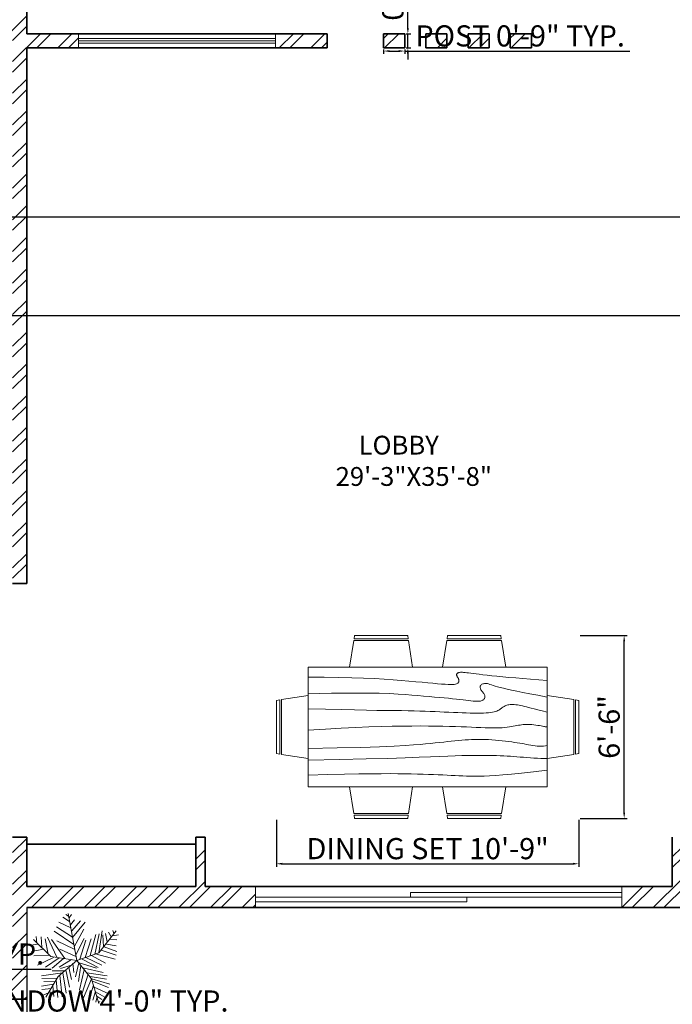
# Model space of a CAD drawing. Units: inches. Extents: x 155 to 1269, y 1260 to 2528.
# Tile 3 of 6: x 514 to 792, y 1484 to 1903. Entities that reach past the tile are written whole.
import ezdxf

# ---------------------------------------------------------------- set-up
doc = ezdxf.new("R2010")
doc.units = ezdxf.units.IN
for name, color, linetype, lineweight in [('A-ANNO-DIMS', 2, 'Continuous', 18), ('A-AREA-IDEN', 7, 'Continuous', 18), ('A-COLS', 7, 'Continuous', 35), ('A-FLOR-EDGE', 7, 'Continuous', 25), ('A-FURN', 8, 'Continuous', 18), ('A-GLAZ', 244, 'Continuous', 18), ('A-WALL', 7, 'Continuous', 35), ('A-WALL-PATT', 252, 'Continuous', 13), ('L-PLNT', 94, 'Continuous', 13)]:
    doc.layers.add(name, color=color, linetype=linetype, lineweight=lineweight)
doc.styles.get("Standard").update_dxf_attribs({"font": 'arial.ttf'})
doc.dimstyles.new('ISO-25', dxfattribs={"dimtxt": 9, "dimasz": 2.5, "dimexe": 1.25, "dimexo": 0.625, "dimtad": 1, "dimlunit": 3, "dimtxsty": 'Standard', "dimcen": 2.5, "dimadec": 0, "dimazin": 0, "dimtfac": 1, "dimtmove": 0, "dimatfit": 3, "dimfxl": 1, "dimarcsym": 0})

# ---------------------------------------------------------------- blocks, each defined once
blk = doc.blocks.new('Dining Set - 36 x 72 in.')
for p, q in [((-22, 27.5), (-22.1562, 26.50042)), ((-22, 27.5), (-6, 27.5)), ((-5.8437, 26.49966), (-6, 27.5)), ((6, 27.5), (5.8438, 26.50042)), ((6, 27.5), (22, 27.5)), ((22.1563, 26.49966), (22, 27.5)), ((-22.2343, 26.00059), (-23.4847, 17.99762)), ((-22.2304, 26), (-5.7608, 26)), ((-5.8416, 26.5), (-22.1534, 26.5)), ((-4.5152, 17.99762), (-5.7655, 25.99926)), ((5.7657, 26.00059), (4.5153, 17.99762)), ((5.7696, 26), (22.2392, 26)), ((22.1584, 26.5), (5.8466, 26.5)), ((23.4848, 17.99762), (22.2345, 25.99926)), ((36, 18), (-36, 18)), ((-36, 18), (-36, -18)), ((36, -18), (36, 18)), ((-44.0006, 8.23428), (-35.9976, 9.48474)), ((44.0006, 8.23428), (35.9976, 9.48474)), ((-45.5, 8), (-44.5004, 8.15617)), ((-45.5, 8), (-45.5, -8)), ((-44.5, -8.15843), (-44.5, 8.15338)), ((-44, 8.23041), (-44, -8.23915)), ((44, 8.23041), (44, -8.23915)), ((44.5, -8.15843), (44.5, 8.15338)), ((45.5, 8), (44.5005, 8.15617)), ((45.5, 8), (45.5, -8)), ((-44.4997, -8.15631), (-45.5, -8)), ((-35.9976, -9.48476), (-43.9993, -8.2345)), ((35.9976, -9.48476), (43.9993, -8.2345)), ((44.4997, -8.15631), (45.5, -8)), ((-36, -18), (36, -18)), ((-22.2343, -26.0006), (-23.4847, -17.99762)), ((-4.5152, -17.99762), (-5.7655, -25.99928)), ((5.7657, -26.0006), (4.5153, -17.99762)), ((23.4848, -17.99762), (22.2345, -25.99928)), ((-22.2304, -26), (-5.7608, -26)), ((-22, -27.5), (-22.1562, -26.50044)), ((-5.8416, -26.5), (-22.1534, -26.5)), ((-5.8437, -26.49967), (-6, -27.5)), ((5.7696, -26), (22.2392, -26)), ((6, -27.5), (5.8438, -26.50044)), ((22.1584, -26.5), (5.8466, -26.5)), ((22.1563, -26.49967), (22, -27.5)), ((-22, -27.5), (-6, -27.5)), ((6, -27.5), (22, -27.5))]:
    blk.add_line(p, q)
for points in [[(-36, 15), (-31.1772, 14.97754), (-26.8079, 14.91406), (-22.8538, 14.81543), (-19.276, 14.6875), (-16.0362, 14.53613), (-13.0957, 14.36718), (-10.4159, 14.18652), (-7.9583, 14), (-5.6904, 13.81315), (-3.6035, 13.63021), (-1.6954, 13.45508), (0.0365, 13.29166), (1.5945, 13.14388), (2.9811, 13.01562), (4.1988, 12.9108), (5.25, 12.83333), (6.1393, 12.78613), (6.8802, 12.76823), (7.4883, 12.77767), (7.9792, 12.8125), (8.3685, 12.87077), (8.6719, 12.95052), (8.9049, 13.0498), (9.0833, 13.16666), (9.2205, 13.29899), (9.3216, 13.44401), (9.3895, 13.59879), (9.4271, 13.76041), (9.4373, 13.92594), (9.4232, 14.09245), (9.3875, 14.257), (9.3333, 14.41666), (9.2638, 14.56917), (9.1836, 14.71484), (9.0975, 14.85465), (9.0104, 14.98958), (8.9272, 15.1206), (8.8529, 15.2487), (8.7922, 15.37483), (8.75, 15.5), (8.7305, 15.62467), (8.7344, 15.74739), (8.7617, 15.86621), (8.8125, 15.97916), (8.8867, 16.08431), (8.9844, 16.17968), (9.1055, 16.26334), (9.25, 16.33333), (9.4189, 16.38802), (9.6172, 16.42708), (9.8506, 16.45052), (10.125, 16.45833), (10.4463, 16.45052), (10.8203, 16.42708), (11.2529, 16.38802), (11.75, 16.33333), (12.3184, 16.26318), (12.9694, 16.17838), (13.7151, 16.07991), (14.5677, 15.96875), (15.5395, 15.84586), (16.6426, 15.71224), (17.8893, 15.56884), (19.2917, 15.41666), (20.859, 15.25667), (22.5879, 15.08984), (24.4721, 14.91715), (26.5052, 14.73958), (28.6809, 14.5581), (30.9929, 14.3737), (33.4347, 14.18733), (36, 14)], [(-36, 10), (-28.9766, 10.14274), (-23.1725, 10.20442), (-18.4241, 10.19775), (-14.5677, 10.13541), (-11.4399, 10.03011), (-8.877, 9.89453), (-6.7154, 9.74137), (-4.7917, 9.58333), (-2.9698, 9.43082), (-1.2246, 9.28515), (0.4415, 9.14534), (2.026, 9.01041), (3.5266, 8.87939), (4.9408, 8.7513), (6.266, 8.62516), (7.5, 8.5), (8.6411, 8.37549), (9.6914, 8.2539), (10.6538, 8.13818), (11.5312, 8.03125), (12.3267, 7.93603), (13.043, 7.85547), (13.6831, 7.79248), (14.25, 7.75), (14.7471, 7.7303), (15.1797, 7.73307), (15.5537, 7.75732), (15.875, 7.80208), (16.1494, 7.86637), (16.3828, 7.94922), (16.5811, 8.04964), (16.75, 8.16666), (16.8944, 8.29915), (17.0143, 8.44531), (17.1089, 8.60319), (17.1771, 8.77083), (17.218, 8.94629), (17.2305, 9.1276), (17.2137, 9.31282), (17.1667, 9.5), (17.0895, 9.6875), (16.987, 9.875), (16.8649, 10.0625), (16.7292, 10.25), (16.5856, 10.4375), (16.4401, 10.625), (16.2985, 10.8125), (16.1667, 11), (16.05, 11.18733), (15.9518, 11.3737), (15.8752, 11.5581), (15.8229, 11.73958), (15.798, 11.91715), (15.8034, 12.08984), (15.842, 12.25667), (15.9167, 12.41666), (16.0295, 12.56836), (16.1784, 12.70833), (16.3605, 12.83268), (16.5729, 12.9375), (16.8127, 13.01888), (17.0768, 13.07291), (17.3625, 13.0957), (17.6667, 13.08333), (17.9894, 13.03312), (18.3418, 12.94726), (18.7382, 12.82918), (19.1927, 12.68229), (19.7195, 12.51001), (20.3327, 12.31575), (21.0465, 12.10294), (21.875, 11.875), (22.8357, 11.63354), (23.959, 11.37304), (25.2786, 11.08618), (26.8282, 10.76562), (28.6414, 10.40405), (30.752, 9.99414), (33.1936, 9.52856), (36, 9)], [(-36, 5.5), (-30.7157, 5.3348), (-26.069, 5.20963), (-21.9946, 5.11767), (-18.4271, 5.05208), (-15.3009, 5.00602), (-12.5508, 4.97265), (-10.1112, 4.94515), (-7.9167, 4.91666), (-5.909, 4.88167), (-4.0586, 4.83984), (-2.3429, 4.79215), (-0.7396, 4.73958), (0.7739, 4.6831), (2.22, 4.6237), (3.6213, 4.56233), (5, 4.5), (6.373, 4.43782), (7.7344, 4.3776), (9.0723, 4.32129), (10.375, 4.27083), (11.6309, 4.22819), (12.8281, 4.19531), (13.9551, 4.17415), (15, 4.16666), (15.954, 4.17448), (16.819, 4.19791), (17.6001, 4.23698), (18.3021, 4.29166), (18.9299, 4.36198), (19.4883, 4.44791), (19.9823, 4.54948), (20.4167, 4.66666), (20.7969, 4.79899), (21.1302, 4.94401), (21.4245, 5.09879), (21.6875, 5.26041), (21.9271, 5.42594), (22.1511, 5.59245), (22.3672, 5.757), (22.5834, 5.91666), (22.8065, 6.06868), (23.0404, 6.21093), (23.2879, 6.34147), (23.5521, 6.45833), (23.8358, 6.55957), (24.142, 6.64323), (24.4735, 6.70735), (24.8334, 6.75), (25.2235, 6.76969), (25.642, 6.76692), (26.0858, 6.74267), (26.5521, 6.69791), (27.0379, 6.63362), (27.5404, 6.55078), (28.0565, 6.45036), (28.5834, 6.33333), (29.1242, 6.19987), (29.7071, 6.04687), (30.3661, 5.87044), (31.1354, 5.66666), (32.0493, 5.43164), (33.142, 5.16146), (34.4475, 4.85221), (36, 4.5)], [(-36, -1), (-30.7915, -0.6591), (-26.0195, -0.38216), (-21.6519, -0.16284), (-17.6563, 0.00521), (-14.0005, 0.12833), (-10.6523, 0.21289), (-7.5796, 0.26522), (-4.75, 0.29166), (-2.134, 0.29793), (0.2878, 0.28711), (2.5317, 0.26163), (4.6146, 0.22396), (6.5529, 0.17651), (8.3633, 0.12174), (10.0623, 0.06209), (11.6667, 0), (13.1899, -0.06201), (14.6341, -0.1211), (15.9982, -0.17432), (17.2813, -0.21875), (18.4823, -0.25147), (19.6003, -0.26953), (20.6343, -0.27002), (21.5834, -0.25), (22.4481, -0.20768), (23.2357, -0.14584), (23.9549, -0.06836), (24.6146, 0.02083), (25.2235, 0.11784), (25.7904, 0.21875), (26.3241, 0.31966), (26.8334, 0.41666), (27.3265, 0.50618), (27.8099, 0.58593), (28.2894, 0.65397), (28.7709, 0.70833), (29.2601, 0.74707), (29.763, 0.76823), (30.2855, 0.76985), (30.8334, 0.75), (31.4088, 0.70784), (31.9994, 0.64713), (32.589, 0.57275), (33.1615, 0.48958), (33.7008, 0.4025), (34.1908, 0.3164), (34.6153, 0.23616), (34.9584, 0.16666), (35.2099, 0.11165), (35.3848, 0.07031), (35.504, 0.04069), (35.5886, 0.02083), (35.6594, 0.00879), (35.7377, 0.0026), (35.8442, 0.00032), (36, 0)], [(-36, -6.5), (-27.1843, -6.31267), (-20.084, -6.1263), (-14.469, -5.9419), (-10.1094, -5.76042), (-6.7752, -5.58285), (-4.2363, -5.41016), (-2.2629, -5.24333), (-0.625, -5.08334), (0.8708, -4.93099), (2.2715, -4.78646), (3.5872, -4.64974), (4.8281, -4.52084), (6.0046, -4.39974), (7.127, -4.28646), (8.2053, -4.18099), (9.25, -4.08334), (10.2705, -3.99382), (11.2734, -3.91407), (12.2647, -3.84603), (13.25, -3.79167), (14.2354, -3.75293), (15.2266, -3.73177), (16.2295, -3.73015), (17.25, -3.75), (18.2912, -3.79248), (19.3451, -3.85547), (20.4009, -3.93604), (21.4479, -4.03125), (22.4754, -4.13819), (23.4727, -4.25391), (24.4289, -4.37549), (25.3334, -4.5), (26.1785, -4.62492), (26.9694, -4.74935), (27.7145, -4.87281), (28.4219, -4.99479), (29.1, -5.11483), (29.7572, -5.23242), (30.4016, -5.34709), (31.0417, -5.45834), (31.6837, -5.56437), (32.3262, -5.65821), (32.9658, -5.73153), (33.599, -5.77604), (34.2224, -5.78345), (34.8327, -5.74545), (35.4264, -5.65373), (36, -5.5)], [(-36, -10), (-26.4022, -9.81299), (-18.4675, -9.62891), (-11.9839, -9.45069), (-6.7396, -9.28125), (-2.5226, -9.12354), (0.8789, -8.98047), (3.6769, -8.85498), (6.0833, -8.75), (8.2767, -8.66765), (10.3021, -8.60677), (12.1712, -8.56543), (13.8958, -8.54167), (15.4876, -8.53353), (16.9583, -8.53907), (18.3197, -8.55632), (19.5834, -8.58334), (20.7616, -8.61841), (21.8685, -8.66081), (22.9188, -8.71004), (23.9271, -8.76563), (24.9081, -8.82707), (25.8763, -8.89388), (26.8465, -8.96558), (27.8334, -9.04167), (28.8474, -9.12118), (29.8828, -9.20117), (30.93, -9.27824), (31.9792, -9.34896), (33.0205, -9.40991), (34.0443, -9.45768), (35.0407, -9.48885), (36, -9.5)], [(-36, -14.5), (-30.0881, -14.33513), (-25.0332, -14.21224), (-20.7312, -14.12647), (-17.0781, -14.07292), (-13.97, -14.04671), (-11.3027, -14.04297), (-8.9724, -14.05681), (-6.875, -14.08334), (-4.9224, -14.11833), (-3.0905, -14.16016), (-1.3709, -14.20785), (0.2448, -14.26042), (1.7647, -14.3169), (3.1973, -14.3763), (4.5507, -14.43767), (5.8333, -14.5), (7.0554, -14.5621), (8.235, -14.62175), (9.3922, -14.67652), (10.5469, -14.72396), (11.7192, -14.76164), (12.929, -14.78711), (14.1965, -14.79794), (15.5417, -14.79167), (16.9933, -14.76424), (18.6152, -14.70508), (20.4804, -14.60197), (22.6615, -14.44271), (25.2312, -14.21509), (28.2624, -13.9069), (31.8277, -13.50594), (36, -13)]]:
    blk.add_lwpolyline(points)
blk = doc.blocks.new('*U11')
for p, q in [((-8.737, 47.138), (-17.069, 52.711)), ((-10.186, 53.64), (-13.084, 55.962)), ((0, 0), (-10.5, 57)), ((-9.099, 51.782), (-6.563, 55.962)), ((-7.65, 43.423), (-2.578, 49.46)), ((-5.839, 35.992), (4.667, 48.067)), ((-5.114, 28.097), (-24.676, 40.636)), ((-7.288, 39.707), (-21.778, 46.673)), ((-5.114, 27.632), (10.463, 46.673)), ((-2.941, 16.486), (8.652, 37.85)), ((27, 9), (48, 36)), ((27.127, 9.056), (31.112, 35.992)), ((44.153, 36.456), (45.239, 32.741)), ((-31.5, 4.5), (-52.5, 25.5)), ((-48.585, 21.131), (-49.309, 29.026)), ((-43.513, 28.561), (-42.427, 15.558)), ((-38.442, 26.239), (-34.819, 7.663)), ((-35.544, 28.097), (-24.314, 3.947)), ((-14.533, 2.09), (-30.834, 25.31)), ((-3.665, 19.273), (-27.574, 35.527)), ((-1.129, 6.734), (9.014, 26.704)), ((3.942, 1.625), (11.187, 24.381)), ((10.101, 3.483), (17.708, 26.239)), ((16.259, 5.805), (23.142, 31.348)), ((22.055, 7.198), (27.489, 32.277)), ((31.836, 30.883), (32.561, 16.486)), ((35.096, 32.741), (37.27, 22.524)), ((38.719, 34.134), (41.979, 28.561)), ((40.53, 25.775), (48.862, 24.846)), ((43.791, 29.954), (51.036, 30.883)), ((-47.498, 19.737), (-55.83, 18.344)), ((-40.615, 13.7), (-55.105, 10.913)), ((-24.314, 23.917), (-2.941, 13.7)), ((-20.691, 13.7), (-1.129, 4.876)), ((29.662, 12.307), (48.137, 6.269)), ((33.285, 16.486), (48.862, 10.913)), ((36.183, 19.737), (48.137, 17.88)), ((-33.37, 6.269), (-52.207, 5.34)), ((-28.299, 3.483), (-47.86, -5.805)), ((-21.416, 3.018), (-38.079, -8.128)), ((0, 0), (-31.5, 4.5)), ((-15.982, 2.09), (-30.11, -9.521)), ((0, 0), (-22.5, -19.5)), ((-6.563, 1.161), (-21.416, -8.128)), ((0, 0), (27, 9)), ((0, 0), (18, -22.5)), ((6.478, 1.625), (26.04, -8.592)), ((11.187, 3.483), (30.749, -5.805)), ((18.07, 5.805), (35.096, -3.483)), ((24.229, 7.663), (46.688, 1.625)), ((-6.563, -5.805), (-19.967, -9.985)), ((-13.446, -11.378), (-8.737, -32.741)), ((-9.461, -8.592), (-6.201, -23.453)), ((-4.752, -3.483), (-3.665, -14.629)), ((2.493, -3.019), (-1.491, -20.202)), ((1.769, -2.555), (24.229, -9.521)), ((5.029, -6.27), (2.131, -25.775)), ((9.014, -11.378), (3.58, -35.992)), ((7.565, -9.056), (32.198, -14.629)), ((-17.431, -15.094), (-42.789, -18.809)), ((-24.314, -21.596), (-42.427, -22.06)), ((-22.5, -19.5), (-37.5, -45)), ((-15.257, -12.772), (-30.11, -12.772)), ((-25.038, -23.918), (-22.865, -45.281)), ((-20.691, -18.345), (-17.793, -44.352)), ((-17.069, -15.094), (-12.721, -40.172)), ((14.085, -16.951), (6.478, -40.172)), ((18.07, -22.524), (8.289, -45.745)), ((12.274, -15.094), (36.907, -18.809)), ((16.259, -19.738), (36.183, -22.989)), ((18, -22.5), (27, -52.5)), ((18.433, -22.524), (40.53, -29.026)), ((-28.299, -29.026), (-42.789, -31.348)), ((-30.834, -34.135), (-42.427, -35.528)), ((-26.849, -26.24), (-40.253, -25.775)), ((-29.023, -30.884), (-27.936, -43.887)), ((20.244, -30.419), (15.897, -44.816)), ((19.157, -25.311), (38.719, -33.206)), ((21.331, -32.741), (39.081, -40.636)), ((-34.457, -39.708), (-40.978, -42.494)), ((-32.646, -36.921), (-31.921, -44.352)), ((22.78, -37.85), (19.519, -48.532)), ((22.78, -38.314), (34.372, -44.816)), ((24.591, -45.745), (23.142, -50.854)), ((24.591, -43.423), (30.749, -47.603)), ((26.764, -49.925), (28.213, -50.854))]:
    blk.add_line(p, q)
blk = doc.blocks.new('POST-9X6')
for p, q in [((0, 0), (0, 6)), ((0, 6), (9, 6)), ((9, 0), (9, 6)), ((0, 0), (9, 0))]:
    blk.add_line(p, q)
blk = doc.blocks.new('*D26')
at = {"layer": 'A-ANNO-DIMS', "color": 0, "lineweight": -2, "transparency": 16777216}
for p, q in [((669.4, 1890.56), (669.4, 1888.58)), ((678.4, 1890.56), (678.4, 1888.58)), ((671.9, 1889.83), (675.9, 1889.83)), ((678.4, 1889.83), (774.28, 1889.83))]:
    blk.add_line(p, q, dxfattribs=at)
at = {"layer": 'A-ANNO-DIMS', "color": 0, "transparency": 16777216}
for points in [[(671.9, 1890.25), (671.9, 1889.41), (669.4, 1889.83)], [(675.9, 1890.25), (675.9, 1889.41), (678.4, 1889.83)]]:
    blk.add_solid(points, dxfattribs=at)
at = {"layer": 'Defpoints', "color": 0, "transparency": 16777216}
for p in [(669.4, 1891.18), (678.4, 1891.18), (678.4, 1889.83)]:
    blk.add_point(p, dxfattribs=at)
at = {"layer": 'A-ANNO-DIMS', "color": 0, "transparency": 16777216, "insert": (727.59, 1895.11), "char_height": 9, "attachment_point": 5}
blk.add_mtext('POST 0\'-9" TYP.', dxfattribs=at)
blk = doc.blocks.new('*D27')
at = {"layer": 'A-ANNO-DIMS', "color": 0, "lineweight": -2, "transparency": 16777216}
for p, q in [((679.75, 1899.68), (679.75, 1958.29)), ((679.02, 1897.18), (681, 1897.18)), ((679.75, 1891.18), (679.75, 1897.18)), ((679.02, 1891.18), (681, 1891.18)), ((679.75, 1888.68), (679.75, 1886.18))]:
    blk.add_line(p, q, dxfattribs=at)
at = {"layer": 'A-ANNO-DIMS', "color": 0, "transparency": 16777216}
for points in [[(679.33, 1899.68), (680.16, 1899.68), (679.75, 1897.18)], [(679.33, 1888.68), (680.16, 1888.68), (679.75, 1891.18)]]:
    blk.add_solid(points, dxfattribs=at)
at = {"layer": 'Defpoints', "color": 0, "transparency": 16777216}
for p in [(678.4, 1897.18), (679.75, 1897.18), (678.4, 1891.18)]:
    blk.add_point(p, dxfattribs=at)
at = {"layer": 'A-ANNO-DIMS', "color": 0, "transparency": 16777216, "insert": (674.53, 1930.24), "char_height": 9, "attachment_point": 5, "rotation": 90}
blk.add_mtext('0\'-6" TYP.', dxfattribs=at)
blk = doc.blocks.new('*D34')
at = {"layer": 'A-ANNO-DIMS', "color": 0, "lineweight": -2, "transparency": 16777216}
for p, q in [((440.63, 1485.56), (440.63, 1477.73)), ((488.63, 1485.56), (488.63, 1477.73)), ((443.13, 1478.98), (486.13, 1478.98)), ((488.63, 1478.98), (606.27, 1478.98))]:
    blk.add_line(p, q, dxfattribs=at)
at = {"layer": 'A-ANNO-DIMS', "color": 0, "transparency": 16777216}
for points in [[(443.13, 1479.4), (443.13, 1478.56), (440.63, 1478.98)], [(486.13, 1479.4), (486.13, 1478.56), (488.63, 1478.98)]]:
    blk.add_solid(points, dxfattribs=at)
at = {"layer": 'Defpoints', "color": 0, "transparency": 16777216}
for p in [(440.63, 1486.18), (488.63, 1486.18), (488.63, 1478.98)]:
    blk.add_point(p, dxfattribs=at)
at = {"layer": 'A-ANNO-DIMS', "color": 0, "transparency": 16777216, "insert": (548.7, 1484.26), "char_height": 9, "attachment_point": 5}
blk.add_mtext('WINDOW 4\'-0" TYP.', dxfattribs=at)
blk = doc.blocks.new('*D36')
at = {"layer": 'A-ANNO-DIMS', "color": 0, "lineweight": -2, "transparency": 16777216}
for p, q in [((373.64, 1500.1), (373.64, 1497.76)), ((376.14, 1499.01), (382.53, 1499.01)), ((385.03, 1500.1), (385.03, 1497.76)), ((385.03, 1499.01), (527.79, 1499.01))]:
    blk.add_line(p, q, dxfattribs=at)
at = {"layer": 'A-ANNO-DIMS', "color": 0, "transparency": 16777216}
for points in [[(376.14, 1499.43), (376.14, 1498.6), (373.64, 1499.01)], [(382.53, 1499.43), (382.53, 1498.6), (385.03, 1499.01)]]:
    blk.add_solid(points, dxfattribs=at)
at = {"layer": 'Defpoints', "color": 0, "transparency": 16777216}
for p in [(373.64, 1500.72), (385.03, 1500.72), (385.03, 1499.01)]:
    blk.add_point(p, dxfattribs=at)
at = {"layer": 'A-ANNO-DIMS', "color": 0, "transparency": 16777216, "insert": (457.66, 1504.29), "char_height": 9, "attachment_point": 5}
blk.add_mtext('BURNER 0\'-11 1/2" TYP.', dxfattribs=at)
blk = doc.blocks.new('*D40')
at = {"layer": 'A-ANNO-DIMS', "color": 0, "lineweight": -2, "transparency": 16777216}
for p, q in [((623.78, 1562.54), (623.78, 1542.59)), ((752.57, 1562.54), (752.57, 1542.59)), ((626.28, 1543.84), (750.07, 1543.84))]:
    blk.add_line(p, q, dxfattribs=at)
at = {"layer": 'A-ANNO-DIMS', "color": 0, "transparency": 16777216}
for points in [[(626.28, 1544.26), (626.28, 1543.43), (623.78, 1543.84)], [(750.07, 1544.26), (750.07, 1543.43), (752.57, 1543.84)]]:
    blk.add_solid(points, dxfattribs=at)
at = {"layer": 'Defpoints', "color": 0, "transparency": 16777216}
for p in [(623.78, 1563.16), (752.57, 1563.16), (752.57, 1543.84)]:
    blk.add_point(p, dxfattribs=at)
at = {"layer": 'A-ANNO-DIMS', "color": 0, "transparency": 16777216, "insert": (688.18, 1549.12), "char_height": 9, "attachment_point": 5}
blk.add_mtext('DINING SET 10\'-9"', dxfattribs=at)
blk = doc.blocks.new('*D41')
at = {"layer": 'A-ANNO-DIMS', "color": 0, "lineweight": -2, "transparency": 16777216}
for p, q in [((753.19, 1641), (773.13, 1641)), ((771.88, 1565.66), (771.88, 1638.5)), ((753.19, 1563.16), (773.13, 1563.16))]:
    blk.add_line(p, q, dxfattribs=at)
at = {"layer": 'A-ANNO-DIMS', "color": 0, "transparency": 16777216}
for points in [[(771.47, 1638.5), (772.3, 1638.5), (771.88, 1641)], [(771.47, 1565.66), (772.3, 1565.66), (771.88, 1563.16)]]:
    blk.add_solid(points, dxfattribs=at)
at = {"layer": 'Defpoints', "color": 0, "transparency": 16777216}
for p in [(752.57, 1641), (771.88, 1641), (752.57, 1563.16)]:
    blk.add_point(p, dxfattribs=at)
at = {"layer": 'A-ANNO-DIMS', "color": 0, "transparency": 16777216, "insert": (766.66, 1602.08), "char_height": 9, "attachment_point": 5, "rotation": 90}
blk.add_mtext('6\'-6"', dxfattribs=at)
blk = doc.blocks.new('*D46')
at = {"layer": 'A-ANNO-DIMS', "color": 0, "lineweight": -2, "transparency": 16777216}
for p, q in [((1009.77, 1819.18), (164.8, 1819.18)), ((166.05, 1779.68), (166.05, 1816.68)), ((1015.06, 1777.18), (164.8, 1777.18))]:
    blk.add_line(p, q, dxfattribs=at)
at = {"layer": 'A-ANNO-DIMS', "color": 0, "transparency": 16777216}
for points in [[(165.63, 1816.68), (166.46, 1816.68), (166.05, 1819.18)], [(165.63, 1779.68), (166.46, 1779.68), (166.05, 1777.18)]]:
    blk.add_solid(points, dxfattribs=at)
at = {"layer": 'Defpoints', "color": 0, "transparency": 16777216}
for p in [(166.05, 1819.18), (1010.4, 1819.18), (1015.68, 1777.18)]:
    blk.add_point(p, dxfattribs=at)
at = {"layer": 'A-ANNO-DIMS', "color": 0, "transparency": 16777216, "insert": (160.82, 1798.18), "char_height": 9, "attachment_point": 5, "rotation": 90}
blk.add_mtext('3\'-6"', dxfattribs=at)

msp = doc.modelspace()

# ---------------------------------------------------------------- hatches: boundary and pattern name
at = {"layer": 'A-WALL-PATT'}
h = msp.add_hatch(dxfattribs=at)
h.set_pattern_fill('ANSI32', color=256)
h.paths.add_polyline_path([(614.897, 1534.181), (593.397, 1534.181), (593.397, 1555.181), (589.397, 1555.181), (589.397, 1534.181), (517.397, 1534.181), (517.397, 1555.181), (511.397, 1555.181), (511.397, 1495.181), (488.631, 1495.181), (488.631, 1486.181), (517.397, 1486.181), (517.397, 1525.181), (614.897, 1525.181)])
h.paths.add_polyline_path([(440.631, 1495.181), (344.954, 1495.181), (344.954, 1486.181), (440.631, 1486.181)])
h.paths.add_polyline_path([(323.954, 1495.181), (302.397, 1495.181), (302.397, 1625.863), (332.397, 1625.863), (332.397, 1631.863), (302.397, 1631.863), (302.397, 1634.984), (293.397, 1634.984), (293.397, 1486.181), (323.954, 1486.181)])
h.paths.add_polyline_path([(302.397, 1753.181), (386.397, 1753.181), (386.397, 1726.181), (392.397, 1726.181), (392.397, 1753.181), (511.397, 1753.181), (511.397, 1693.181), (392.397, 1693.181), (392.397, 1696.181), (386.397, 1696.181), (386.397, 1693.181), (368.397, 1693.181), (368.397, 1687.181), (511.397, 1687.181), (511.397, 1663.181), (517.397, 1663.181), (517.397, 1891.181), (539.397, 1891.181), (539.397, 1897.181), (517.397, 1897.181), (517.397, 2050.181), (511.397, 2050.181), (511.397, 1903.181), (374.397, 1903.181), (374.397, 1897.181), (410.397, 1897.181), (410.397, 1843.181), (416.397, 1843.181), (416.397, 1897.181), (511.397, 1897.181), (511.397, 1759.181), (416.397, 1759.181), (416.397, 1813.181), (410.397, 1813.181), (410.397, 1759.181), (302.397, 1759.181), (302.397, 1897.181), (338.397, 1897.181), (338.397, 1903.181), (302.397, 1903.181), (302.397, 1935.29), (293.397, 1935.29), (293.397, 1682.984), (302.397, 1682.984), (302.397, 1687.181), (338.397, 1687.181), (338.397, 1693.181), (302.397, 1693.181)])
h.paths.add_polyline_path([(645.397, 1897.181), (623.397, 1897.181), (623.397, 1891.181), (645.397, 1891.181)])
h.paths.add_polyline_path([(678.397, 1897.181), (669.397, 1897.181), (669.397, 1891.181), (678.397, 1891.181)])
h.paths.add_polyline_path([(696.397, 1897.181), (687.397, 1897.181), (687.397, 1891.181), (696.397, 1891.181)])
h.paths.add_polyline_path([(714.397, 1897.181), (705.397, 1897.181), (705.397, 1891.181), (714.397, 1891.181)])
h.paths.add_polyline_path([(732.397, 1897.181), (723.397, 1897.181), (723.397, 1891.181), (732.397, 1891.181)])
h.paths.add_polyline_path([(302.397, 2033.891), (293.397, 2033.891), (293.397, 1959.29), (302.397, 1959.29)], flags=17)
h.paths.add_polyline_path([(302.397, 2089.181), (511.397, 2089.181), (511.397, 2086.181), (517.397, 2086.181), (517.397, 2089.181), (527.397, 2089.181), (527.397, 2095.181), (302.397, 2095.181), (302.397, 2145.471), (293.397, 2145.471), (293.397, 2057.891), (302.397, 2057.891)])
h.paths.add_polyline_path([(773.397, 2095.181), (572.397, 2095.181), (572.397, 2308.181), (613.397, 2308.181), (613.397, 2443.181), (557.897, 2443.181), (557.897, 2434.181), (604.397, 2434.181), (604.397, 2314.181), (490.397, 2314.181), (490.397, 2359.181), (484.397, 2359.181), (484.397, 2314.181), (374.397, 2314.181), (374.397, 2308.181), (566.397, 2308.181), (566.397, 2095.181), (563.397, 2095.181), (563.397, 2089.181), (773.397, 2089.181)])
h.paths.add_polyline_path([(1070.397, 2147.681), (1061.397, 2147.681), (1061.397, 2095.181), (857.397, 2095.181), (857.397, 2089.181), (868.397, 2089.181), (868.397, 2086.181), (874.397, 2086.181), (874.397, 2089.181), (1061.397, 2089.181), (1061.397, 2050.181), (1070.397, 2050.181)])
h.paths.add_polyline_path([(821.397, 2095.181), (818.397, 2095.181), (818.397, 2308.181), (1022.397, 2308.181), (1022.397, 2314.181), (940.397, 2314.181), (940.397, 2434.181), (1077.397, 2434.181), (1077.397, 2389.181), (1083.397, 2389.181), (1083.397, 2434.181), (1129.897, 2434.181), (1129.897, 2443.181), (887.897, 2443.181), (887.897, 2434.181), (934.397, 2434.181), (934.397, 2314.181), (820.397, 2314.181), (820.397, 2359.181), (814.397, 2359.181), (814.397, 2314.181), (809.397, 2314.181), (809.397, 2308.181), (812.397, 2308.181), (812.397, 2095.181), (809.397, 2095.181), (809.397, 2089.181), (821.397, 2089.181)])
h.paths.add_polyline_path([(874.397, 2050.181), (868.397, 2050.181), (868.397, 1741.181), (877.397, 1741.181), (877.397, 1747.181), (892.397, 1747.181), (892.397, 1753.181), (874.397, 1753.181), (874.397, 1819.181), (940.397, 1819.181), (940.397, 1753.181), (922.397, 1753.181), (922.397, 1747.181), (946.397, 1747.181), (946.397, 1819.181), (1151.397, 1819.181), (1151.397, 1683.181), (931.397, 1683.181), (931.397, 1677.181), (1064.397, 1677.181), (1064.397, 1495.181), (877.397, 1495.181), (877.397, 1638.181), (868.397, 1638.181), (868.397, 1534.181), (796.397, 1534.181), (796.397, 1555.181), (792.397, 1555.181), (792.397, 1534.181), (770.897, 1534.181), (770.897, 1525.181), (868.397, 1525.181), (868.397, 1486.181), (1073.397, 1486.181), (1073.397, 1677.181), (1160.397, 1677.181), (1160.397, 1825.181), (1070.397, 1825.181), (1070.397, 1942.181), (1061.397, 1942.181), (1061.397, 1903.181), (913.397, 1903.181), (913.397, 1897.181), (1061.397, 1897.181), (1061.397, 1825.181), (957.406, 1825.181), (957.406, 1861.181), (951.406, 1861.181), (951.406, 1825.181), (874.397, 1825.181), (874.397, 1897.181), (877.397, 1897.181), (877.397, 1903.181), (874.397, 1903.181)])
h.paths.add_polyline_path([(1070.397, 2305.181), (1206.397, 2305.181), (1206.397, 2443.181), (1150.897, 2443.181), (1150.897, 2434.181), (1197.397, 2434.181), (1197.397, 2314.181), (1083.397, 2314.181), (1083.397, 2359.181), (1077.397, 2359.181), (1077.397, 2314.181), (1058.397, 2314.181), (1058.397, 2308.181), (1061.397, 2308.181), (1061.397, 2255.681), (1070.397, 2255.681)])
h.paths.add_polyline_path([(866.897, 2443.181), (673.397, 2443.181), (673.397, 2308.181), (773.397, 2308.181), (773.397, 2314.181), (682.397, 2314.181), (682.397, 2434.181), (814.397, 2434.181), (814.397, 2389.181), (818.897, 2389.181), (820.397, 2389.181), (820.397, 2434.181), (866.897, 2434.181)])
h.paths.add_polyline_path([(536.897, 2443.181), (293.397, 2443.181), (293.397, 2253.471), (302.397, 2253.471), (302.397, 2308.181), (338.397, 2308.181), (338.397, 2314.181), (302.397, 2314.181), (302.397, 2434.181), (484.397, 2434.181), (484.397, 2389.181), (490.397, 2389.181), (490.397, 2434.181), (536.897, 2434.181)])

# ---------------------------------------------------------------- linework, layer by layer
at = {"layer": 'A-FLOR-EDGE'}
msp.add_line((517.397, 1525.181), (517.397, 1384.181), dxfattribs=at)
at = {"layer": 'A-GLAZ'}
for p, q in [((539.397, 1895.181), (623.397, 1895.181)), ((539.397, 1894.181), (623.397, 1894.181)), ((539.397, 1893.181), (623.397, 1893.181)), ((680.897, 1531.681), (770.897, 1531.681)), ((680.897, 1529.681), (680.897, 1531.681)), ((614.897, 1529.681), (770.897, 1529.681)), ((614.897, 1527.681), (704.897, 1527.681)), ((704.897, 1529.681), (704.897, 1527.681))]:
    msp.add_line(p, q, dxfattribs=at)
for points in [[(539.397, 1897.181), (623.397, 1897.181), (623.397, 1891.181), (539.397, 1891.181)], [(614.897, 1534.181), (770.897, 1534.181), (770.897, 1525.181), (614.897, 1525.181)]]:
    msp.add_lwpolyline(points, close=True, dxfattribs=at)
at = {"layer": 'A-WALL'}
for p, q in [((517.397, 2050.181), (517.397, 1897.181)), ((517.397, 1897.181), (645.397, 1897.181)), ((645.397, 1891.181), (645.397, 1897.181)), ((517.397, 1891.181), (645.397, 1891.181)), ((517.397, 1891.181), (517.397, 1663.181)), ((511.397, 1663.181), (517.397, 1663.181)), ((511.397, 1555.181), (517.397, 1555.181)), ((517.397, 1555.181), (517.397, 1534.181)), ((589.397, 1555.181), (589.397, 1534.181)), ((593.397, 1555.181), (589.397, 1555.181)), ((593.397, 1555.181), (593.397, 1534.181)), ((792.397, 1555.181), (792.397, 1534.181)), ((517.397, 1552.181), (589.397, 1552.181)), ((517.397, 1534.181), (589.397, 1534.181)), ((593.397, 1534.181), (792.397, 1534.181)), ((517.397, 1525.181), (868.397, 1525.181)), ((293.397, 1486.181), (517.397, 1486.181))]:
    msp.add_line(p, q, dxfattribs=at)

# ---------------------------------------------------------------- block references
at = {"layer": 'A-COLS'}
for p in [(669.397, 1891.181), (687.397, 1891.181), (705.397, 1891.181), (723.397, 1891.181)]:
    msp.add_blockref('POST-9X6', p, dxfattribs=at)
at = {"layer": 'A-FURN', "xscale": 1.415180641918518, "yscale": 1.415180641918518, "zscale": 1.415180641918518}
msp.add_blockref('Dining Set - 36 x 72 in.', (688.175, 1602.078), dxfattribs=at)
at = {"layer": 'L-PLNT', "xscale": 0.3495173552522817, "yscale": 0.3495173552522817, "zscale": 0.3495173552522817}
msp.add_blockref('*U11', (538.697, 1502.73), dxfattribs=at)

# ---------------------------------------------------------------- texts
at = {"layer": 'A-AREA-IDEN', "insert": (648.997, 1726.059), "char_height": 8, "attachment_point": 1}
msp.add_mtext_dynamic_manual_height_columns('    LOBBY 29\'-3"X35\'-8"', width=63.69718, gutter_width=12.5, heights=[0], dxfattribs=at)

# ---------------------------------------------------------------- dimensions: what is measured, and where the dimension line sits
at = {"layer": 'A-ANNO-DIMS'}
dim = msp.add_linear_dim(base=(679.747, 1897.181), p1=(678.397, 1891.181), p2=(678.397, 1897.181), angle=90, text='<> TYP.', dimstyle='ISO-25', override={"dimdec": 1, "dimlfac": 1, "dimrnd": 0, "dimzin": 1, "dimdsep": 46, "dimlunit": 4, "dimfrac": 2}, dxfattribs=at)
dim.commit()
dim.dimension.update_dxf_attribs({"geometry": '*D27', "text_midpoint": (674.527, 1930.236)})
for base, p1, p2, text, picture, middle in [((678.397, 1889.831), (669.397, 1891.181), (678.397, 1891.181), 'POST <> TYP.', '*D26', (727.591, 1895.112)), ((752.566, 1543.843), (623.785, 1563.16), (752.566, 1563.16), 'DINING SET <>', '*D40', (688.175, 1549.121)), ((385.03, 1499.015), (373.642, 1500.723), (385.03, 1500.723), 'BURNER <> TYP.', '*D36', (457.659, 1504.293)), ((488.631, 1478.981), (440.631, 1486.181), (488.631, 1486.181), 'WINDOW <> TYP.', '*D34', (548.7, 1484.262))]:
    dim = msp.add_linear_dim(base=base, p1=p1, p2=p2, text=text, dimstyle='ISO-25', override={"dimdec": 1, "dimlfac": 1, "dimrnd": 0, "dimzin": 1, "dimdsep": 46, "dimlunit": 4, "dimfrac": 2}, dxfattribs=at)
    dim.commit()
    dim.dimension.update_dxf_attribs({"geometry": picture, "text_midpoint": middle})
for base, p1, p2, picture, middle in [((166.047, 1819.181), (1015.681, 1777.181), (1010.397, 1819.181), '*D46', (160.824, 1798.181)), ((771.883, 1640.995), (752.566, 1563.16), (752.566, 1640.995), '*D41', (766.663, 1602.078))]:
    dim = msp.add_linear_dim(base=base, p1=p1, p2=p2, angle=90, dimstyle='ISO-25', override={"dimdec": 1, "dimlfac": 1, "dimrnd": 0, "dimzin": 1, "dimdsep": 46, "dimlunit": 4, "dimfrac": 2}, dxfattribs=at)
    dim.commit()
    dim.dimension.update_dxf_attribs({"geometry": picture, "text_midpoint": middle})

doc.saveas('drawing.dxf')
